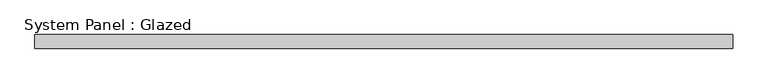
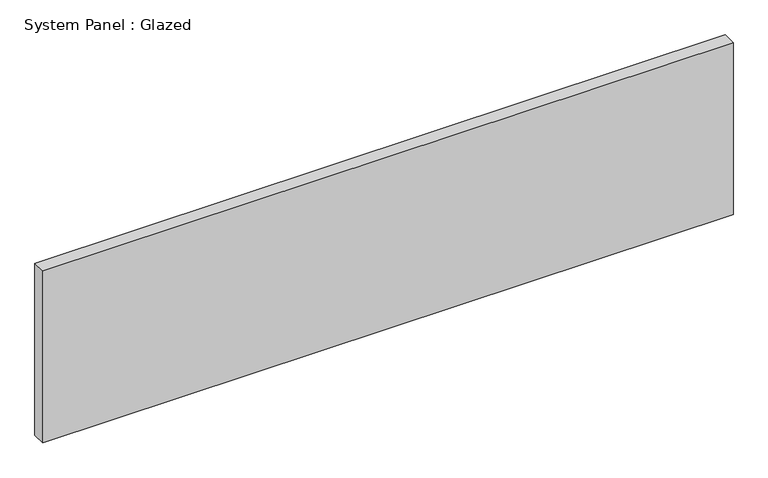
"""IFC4 building model written with IfcOpenShell, lengths in millimetres: plate geometry, System Panel : Glazed."""

from ifc_helpers import new_model, si_unit, origin, origin_with_axes, place, context, project, spatial, polyline, outline, extrude, source, transform, mapped, element, save


def system_panel_glazed_2a12a50e(model_context):
    return source(origin(), model_context, "Body", "SweptSolid", [
        extrude(outline(polyline([(650.8750001, -44.45), (-650.8750001, -44.45), (-650.8750001, -19.05), (650.8750001, -19.05), (650.8750001, -44.45)])), origin_with_axes(), (0.0, 0.0, 1.0), 342.9),
    ])


if __name__ == "__main__":
    model = new_model("IFC4")
    model_context = context("Model", 3, world=origin())
    ifc_project = project(units=[si_unit("LENGTHUNIT", "METRE", prefix="MILLI")], contexts=[model_context])
    site = spatial("IfcSite", under=ifc_project)
    building = spatial("IfcBuilding", under=site)
    placement = place(None, origin())
    system_panel_glazed_shape = system_panel_glazed_2a12a50e(model_context)
    element("IfcPlate", 1, ObjectType="System Panel : Glazed", at=placement, inside=building, context=model_context, shape_type="MappedRepresentation", body=[
        mapped(system_panel_glazed_shape, transform((0.0, 0.0, 0.0), x_axis=(1.0, 0.0, 0.0), y_axis=(0.0, 1.0, 0.0), z_axis=(0.0, 0.0, 1.0))),
    ])
    save(model, "model.ifc")

# Revit data of these elements
# Type "System Panel : Glazed"
#   Construction Type Id = "GSP4R"
#   Analytic Construction = "1/8 in Pilkington single glazing"
#   Visual Light Transmittance = 0.9
#   Solar Heat Gain Coefficient = 0.86
#   Heat Transfer Coefficient (U) = 1.18115 BTU/(h·ft²·°F)
#   Define Thermal Properties by = 1
# Element 1 (IfcPlate, "System Panel : Glazed")
#   Materials on its faces: "glass panel 223"
# Materials
#   "glass panel 223": class "Generic", colour RGB 120 120 120, transparency 0, Cost = 0
